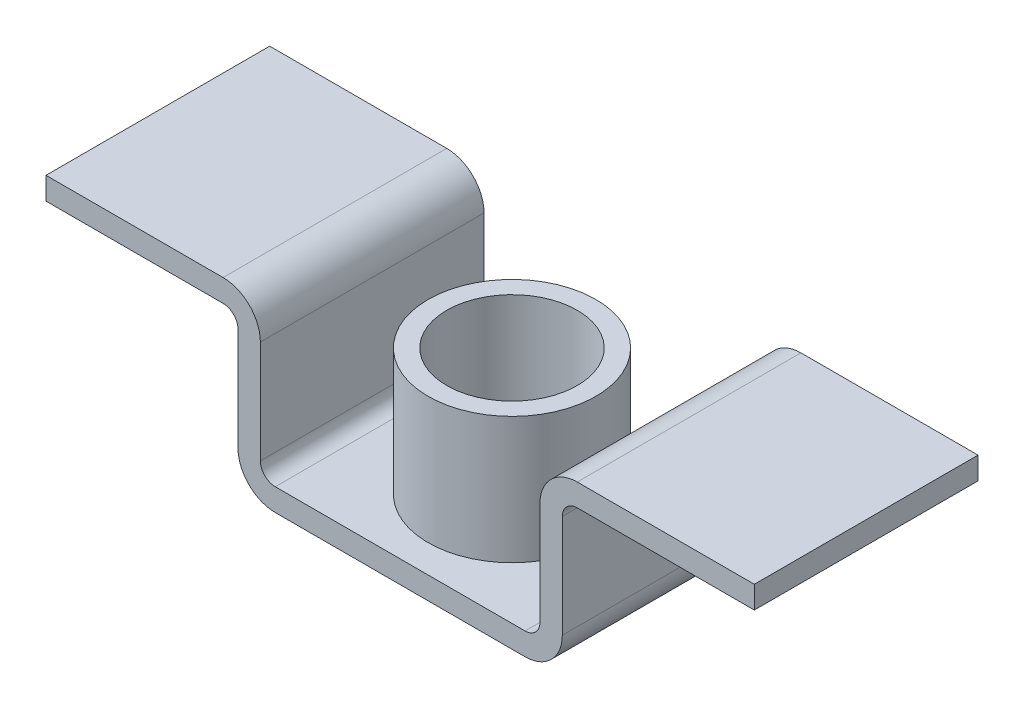
ISO-10303-21;
HEADER;
FILE_DESCRIPTION(('STEP AP214'),'2;1');
FILE_NAME('part.step','',(''),(''),'','','');
FILE_SCHEMA(('AUTOMOTIVE_DESIGN { 1 0 10303 214 1 1 1 1 }'));
ENDSEC;
DATA;
#1=APPLICATION_CONTEXT('core data for automotive mechanical design processes');
#2=APPLICATION_PROTOCOL_DEFINITION('international standard','automotive_design',2000,#1);
#3=PRODUCT_CONTEXT('',#1,'mechanical');
#4=PRODUCT('Part','Part','',(#3));
#5=PRODUCT_RELATED_PRODUCT_CATEGORY('part','',(#4));
#6=PRODUCT_DEFINITION_FORMATION('','',#4);
#7=PRODUCT_DEFINITION_CONTEXT('part definition',#1,'design');
#8=PRODUCT_DEFINITION('design','',#6,#7);
#9=PRODUCT_DEFINITION_SHAPE('','',#8);
#10=(LENGTH_UNIT() NAMED_UNIT(*) SI_UNIT(.MILLI.,.METRE.));
#11=(NAMED_UNIT(*) PLANE_ANGLE_UNIT() SI_UNIT($,.RADIAN.));
#12=(NAMED_UNIT(*) SI_UNIT($,.STERADIAN.) SOLID_ANGLE_UNIT());
#13=UNCERTAINTY_MEASURE_WITH_UNIT(LENGTH_MEASURE(1.E-05),#10,'distance_accuracy_value','');
#14=(GEOMETRIC_REPRESENTATION_CONTEXT(3) GLOBAL_UNCERTAINTY_ASSIGNED_CONTEXT((#13)) GLOBAL_UNIT_ASSIGNED_CONTEXT((#10,
#11,#12)) REPRESENTATION_CONTEXT('',''));
#15=CARTESIAN_POINT('',(0.,0.,0.));
#16=DIRECTION('',(0.,0.,1.));
#17=DIRECTION('',(1.,0.,0.));
#18=AXIS2_PLACEMENT_3D('',#15,#16,#17);
#19=CARTESIAN_POINT('',(-167.5,-188.,150.));
#20=DIRECTION('',(0.,0.,-1.));
#21=DIRECTION('',(-1.,0.,0.));
#22=AXIS2_PLACEMENT_3D('',#19,#20,#21);
#23=CYLINDRICAL_SURFACE('',#22,20.);
#24=CARTESIAN_POINT('',(-167.5,-188.,-150.));
#25=DIRECTION('',(0.,0.,1.));
#26=DIRECTION('',(1.,0.,0.));
#27=AXIS2_PLACEMENT_3D('',#24,#25,#26);
#28=CIRCLE('',#27,20.);
#29=CARTESIAN_POINT('',(-187.5,-188.,-150.));
#30=VERTEX_POINT('',#29);
#31=CARTESIAN_POINT('',(-167.5,-208.,-150.));
#32=VERTEX_POINT('',#31);
#33=EDGE_CURVE('E207',#30,#32,#28,.T.);
#34=ORIENTED_EDGE('',*,*,#33,.F.);
#35=DIRECTION('',(0.,0.,-1.));
#36=VECTOR('',#35,1.);
#37=CARTESIAN_POINT('',(-187.5,-188.,150.));
#38=LINE('',#37,#36);
#39=CARTESIAN_POINT('',(-187.5,-188.,150.));
#40=VERTEX_POINT('',#39);
#41=EDGE_CURVE('E50',#40,#30,#38,.T.);
#42=ORIENTED_EDGE('',*,*,#41,.F.);
#43=CARTESIAN_POINT('',(-167.5,-188.,150.));
#44=DIRECTION('',(0.,0.,1.));
#45=DIRECTION('',(1.,0.,0.));
#46=AXIS2_PLACEMENT_3D('',#43,#44,#45);
#47=CIRCLE('',#46,20.);
#48=CARTESIAN_POINT('',(-167.5,-208.,150.));
#49=VERTEX_POINT('',#48);
#50=EDGE_CURVE('E270',#40,#49,#47,.T.);
#51=ORIENTED_EDGE('',*,*,#50,.T.);
#52=DIRECTION('',(0.,0.,-1.));
#53=VECTOR('',#52,1.);
#54=CARTESIAN_POINT('',(-167.5,-208.,150.));
#55=LINE('',#54,#53);
#56=EDGE_CURVE('E133',#49,#32,#55,.T.);
#57=ORIENTED_EDGE('',*,*,#56,.T.);
#58=EDGE_LOOP('',(#34,#42,#51,#57));
#59=FACE_BOUND('',#58,.T.);
#60=ADVANCED_FACE('F39',(#59),#23,.F.);
#61=CARTESIAN_POINT('',(-187.5,-50.0000000000003,150.));
#62=DIRECTION('',(1.,0.,0.));
#63=DIRECTION('',(0.,1.,0.));
#64=AXIS2_PLACEMENT_3D('',#61,#62,#63);
#65=PLANE('',#64);
#66=DIRECTION('',(0.,-1.,0.));
#67=VECTOR('',#66,1.);
#68=CARTESIAN_POINT('',(-187.5,-50.0000000000003,-150.));
#69=LINE('',#68,#67);
#70=CARTESIAN_POINT('',(-187.5,-50.0000000000003,-150.));
#71=VERTEX_POINT('',#70);
#72=EDGE_CURVE('E262',#71,#30,#69,.T.);
#73=ORIENTED_EDGE('',*,*,#72,.F.);
#74=DIRECTION('',(0.,0.,-1.));
#75=VECTOR('',#74,1.);
#76=CARTESIAN_POINT('',(-187.5,-50.0000000000003,150.));
#77=LINE('',#76,#75);
#78=CARTESIAN_POINT('',(-187.5,-50.0000000000003,150.));
#79=VERTEX_POINT('',#78);
#80=EDGE_CURVE('E119',#79,#71,#77,.T.);
#81=ORIENTED_EDGE('',*,*,#80,.F.);
#82=DIRECTION('',(0.,-1.,0.));
#83=VECTOR('',#82,1.);
#84=CARTESIAN_POINT('',(-187.5,-50.0000000000003,150.));
#85=LINE('',#84,#83);
#86=EDGE_CURVE('E200',#79,#40,#85,.T.);
#87=ORIENTED_EDGE('',*,*,#86,.T.);
#88=ORIENTED_EDGE('',*,*,#41,.T.);
#89=EDGE_LOOP('',(#73,#81,#87,#88));
#90=FACE_BOUND('',#89,.T.);
#91=ADVANCED_FACE('F302',(#90),#65,.T.);
#92=CARTESIAN_POINT('',(-237.5,-50.,150.));
#93=DIRECTION('',(0.,0.,-1.));
#94=DIRECTION('',(-1.,0.,0.));
#95=AXIS2_PLACEMENT_3D('',#92,#93,#94);
#96=CYLINDRICAL_SURFACE('',#95,50.);
#97=CARTESIAN_POINT('',(-237.5,-50.,-150.));
#98=DIRECTION('',(0.,0.,-1.));
#99=DIRECTION('',(-1.,0.,0.));
#100=AXIS2_PLACEMENT_3D('',#97,#98,#99);
#101=CIRCLE('',#100,50.);
#102=CARTESIAN_POINT('',(-237.5,0.,-150.));
#103=VERTEX_POINT('',#102);
#104=EDGE_CURVE('E188',#103,#71,#101,.T.);
#105=ORIENTED_EDGE('',*,*,#104,.F.);
#106=DIRECTION('',(0.,0.,-1.));
#107=VECTOR('',#106,1.);
#108=CARTESIAN_POINT('',(-237.5,0.,150.));
#109=LINE('',#108,#107);
#110=CARTESIAN_POINT('',(-237.5,0.,150.));
#111=VERTEX_POINT('',#110);
#112=EDGE_CURVE('E182',#111,#103,#109,.T.);
#113=ORIENTED_EDGE('',*,*,#112,.F.);
#114=CARTESIAN_POINT('',(-237.5,-50.,150.));
#115=DIRECTION('',(0.,0.,-1.));
#116=DIRECTION('',(-1.,0.,0.));
#117=AXIS2_PLACEMENT_3D('',#114,#115,#116);
#118=CIRCLE('',#117,50.);
#119=EDGE_CURVE('E184',#111,#79,#118,.T.);
#120=ORIENTED_EDGE('',*,*,#119,.T.);
#121=ORIENTED_EDGE('',*,*,#80,.T.);
#122=EDGE_LOOP('',(#105,#113,#120,#121));
#123=FACE_BOUND('',#122,.T.);
#124=ADVANCED_FACE('F181',(#123),#96,.T.);
#125=CARTESIAN_POINT('',(-475.,0.,150.));
#126=DIRECTION('',(0.,1.,0.));
#127=DIRECTION('',(0.,0.,1.));
#128=AXIS2_PLACEMENT_3D('',#125,#126,#127);
#129=PLANE('',#128);
#130=DIRECTION('',(1.,0.,0.));
#131=VECTOR('',#130,1.);
#132=CARTESIAN_POINT('',(-475.,0.,-150.));
#133=LINE('',#132,#131);
#134=CARTESIAN_POINT('',(-475.,0.,-150.));
#135=VERTEX_POINT('',#134);
#136=EDGE_CURVE('E261',#135,#103,#133,.T.);
#137=ORIENTED_EDGE('',*,*,#136,.F.);
#138=DIRECTION('',(0.,0.,-1.));
#139=VECTOR('',#138,1.);
#140=CARTESIAN_POINT('',(-475.,0.,150.));
#141=LINE('',#140,#139);
#142=CARTESIAN_POINT('',(-475.,0.,150.));
#143=VERTEX_POINT('',#142);
#144=EDGE_CURVE('E193',#143,#135,#141,.T.);
#145=ORIENTED_EDGE('',*,*,#144,.F.);
#146=DIRECTION('',(1.,0.,0.));
#147=VECTOR('',#146,1.);
#148=CARTESIAN_POINT('',(-475.,0.,150.));
#149=LINE('',#148,#147);
#150=EDGE_CURVE('E197',#143,#111,#149,.T.);
#151=ORIENTED_EDGE('',*,*,#150,.T.);
#152=ORIENTED_EDGE('',*,*,#112,.T.);
#153=EDGE_LOOP('',(#137,#145,#151,#152));
#154=FACE_BOUND('',#153,.T.);
#155=ADVANCED_FACE('F203',(#154),#129,.T.);
#156=CARTESIAN_POINT('',(-475.,-30.,150.));
#157=DIRECTION('',(-1.,0.,0.));
#158=DIRECTION('',(0.,0.,1.));
#159=AXIS2_PLACEMENT_3D('',#156,#157,#158);
#160=PLANE('',#159);
#161=DIRECTION('',(0.,1.,0.));
#162=VECTOR('',#161,1.);
#163=CARTESIAN_POINT('',(-475.,-30.,-150.));
#164=LINE('',#163,#162);
#165=CARTESIAN_POINT('',(-475.,-30.,-150.));
#166=VERTEX_POINT('',#165);
#167=EDGE_CURVE('E256',#166,#135,#164,.T.);
#168=ORIENTED_EDGE('',*,*,#167,.F.);
#169=DIRECTION('',(0.,0.,-1.));
#170=VECTOR('',#169,1.);
#171=CARTESIAN_POINT('',(-475.,-30.,150.));
#172=LINE('',#171,#170);
#173=CARTESIAN_POINT('',(-475.,-30.,150.));
#174=VERTEX_POINT('',#173);
#175=EDGE_CURVE('E271',#174,#166,#172,.T.);
#176=ORIENTED_EDGE('',*,*,#175,.F.);
#177=DIRECTION('',(0.,1.,0.));
#178=VECTOR('',#177,1.);
#179=CARTESIAN_POINT('',(-475.,-30.,150.));
#180=LINE('',#179,#178);
#181=EDGE_CURVE('E205',#174,#143,#180,.T.);
#182=ORIENTED_EDGE('',*,*,#181,.T.);
#183=ORIENTED_EDGE('',*,*,#144,.T.);
#184=EDGE_LOOP('',(#168,#176,#182,#183));
#185=FACE_BOUND('',#184,.T.);
#186=ADVANCED_FACE('F320',(#185),#160,.T.);
#187=CARTESIAN_POINT('',(-237.5,-30.,150.));
#188=DIRECTION('',(0.,-1.,0.));
#189=DIRECTION('',(1.,0.,0.));
#190=AXIS2_PLACEMENT_3D('',#187,#188,#189);
#191=PLANE('',#190);
#192=DIRECTION('',(-1.,0.,0.));
#193=VECTOR('',#192,1.);
#194=CARTESIAN_POINT('',(-237.5,-30.,-150.));
#195=LINE('',#194,#193);
#196=CARTESIAN_POINT('',(-237.5,-30.,-150.));
#197=VERTEX_POINT('',#196);
#198=EDGE_CURVE('E254',#197,#166,#195,.T.);
#199=ORIENTED_EDGE('',*,*,#198,.F.);
#200=DIRECTION('',(0.,0.,-1.));
#201=VECTOR('',#200,1.);
#202=CARTESIAN_POINT('',(-237.5,-30.,150.));
#203=LINE('',#202,#201);
#204=CARTESIAN_POINT('',(-237.5,-30.,150.));
#205=VERTEX_POINT('',#204);
#206=EDGE_CURVE('E272',#205,#197,#203,.T.);
#207=ORIENTED_EDGE('',*,*,#206,.F.);
#208=DIRECTION('',(-1.,0.,0.));
#209=VECTOR('',#208,1.);
#210=CARTESIAN_POINT('',(-237.5,-30.,150.));
#211=LINE('',#210,#209);
#212=EDGE_CURVE('E204',#205,#174,#211,.T.);
#213=ORIENTED_EDGE('',*,*,#212,.T.);
#214=ORIENTED_EDGE('',*,*,#175,.T.);
#215=EDGE_LOOP('',(#199,#207,#213,#214));
#216=FACE_BOUND('',#215,.T.);
#217=ADVANCED_FACE('F319',(#216),#191,.T.);
#218=CARTESIAN_POINT('',(-237.5,-50.,150.));
#219=DIRECTION('',(0.,0.,-1.));
#220=DIRECTION('',(-1.,0.,0.));
#221=AXIS2_PLACEMENT_3D('',#218,#219,#220);
#222=CYLINDRICAL_SURFACE('',#221,20.);
#223=CARTESIAN_POINT('',(-237.5,-50.,-150.));
#224=DIRECTION('',(0.,0.,1.));
#225=DIRECTION('',(1.,0.,0.));
#226=AXIS2_PLACEMENT_3D('',#223,#224,#225);
#227=CIRCLE('',#226,20.);
#228=CARTESIAN_POINT('',(-217.5,-50.0000000000001,-150.));
#229=VERTEX_POINT('',#228);
#230=EDGE_CURVE('E252',#229,#197,#227,.T.);
#231=ORIENTED_EDGE('',*,*,#230,.F.);
#232=DIRECTION('',(0.,0.,-1.));
#233=VECTOR('',#232,1.);
#234=CARTESIAN_POINT('',(-217.5,-50.0000000000001,150.));
#235=LINE('',#234,#233);
#236=CARTESIAN_POINT('',(-217.5,-50.0000000000001,150.));
#237=VERTEX_POINT('',#236);
#238=EDGE_CURVE('E274',#237,#229,#235,.T.);
#239=ORIENTED_EDGE('',*,*,#238,.F.);
#240=CARTESIAN_POINT('',(-237.5,-50.,150.));
#241=DIRECTION('',(0.,0.,1.));
#242=DIRECTION('',(1.,0.,0.));
#243=AXIS2_PLACEMENT_3D('',#240,#241,#242);
#244=CIRCLE('',#243,20.);
#245=EDGE_CURVE('E460',#237,#205,#244,.T.);
#246=ORIENTED_EDGE('',*,*,#245,.T.);
#247=ORIENTED_EDGE('',*,*,#206,.T.);
#248=EDGE_LOOP('',(#231,#239,#246,#247));
#249=FACE_BOUND('',#248,.T.);
#250=ADVANCED_FACE('F322',(#249),#222,.F.);
#251=CARTESIAN_POINT('',(-217.5,-188.,150.));
#252=DIRECTION('',(-1.,0.,0.));
#253=DIRECTION('',(0.,0.,1.));
#254=AXIS2_PLACEMENT_3D('',#251,#252,#253);
#255=PLANE('',#254);
#256=DIRECTION('',(0.,1.,0.));
#257=VECTOR('',#256,1.);
#258=CARTESIAN_POINT('',(-217.5,-188.,-150.));
#259=LINE('',#258,#257);
#260=CARTESIAN_POINT('',(-217.5,-188.,-150.));
#261=VERTEX_POINT('',#260);
#262=EDGE_CURVE('E247',#261,#229,#259,.T.);
#263=ORIENTED_EDGE('',*,*,#262,.F.);
#264=DIRECTION('',(0.,0.,-1.));
#265=VECTOR('',#264,1.);
#266=CARTESIAN_POINT('',(-217.5,-188.,150.));
#267=LINE('',#266,#265);
#268=CARTESIAN_POINT('',(-217.5,-188.,150.));
#269=VERTEX_POINT('',#268);
#270=EDGE_CURVE('E280',#269,#261,#267,.T.);
#271=ORIENTED_EDGE('',*,*,#270,.F.);
#272=DIRECTION('',(0.,1.,0.));
#273=VECTOR('',#272,1.);
#274=CARTESIAN_POINT('',(-217.5,-188.,150.));
#275=LINE('',#274,#273);
#276=EDGE_CURVE('E452',#269,#237,#275,.T.);
#277=ORIENTED_EDGE('',*,*,#276,.T.);
#278=ORIENTED_EDGE('',*,*,#238,.T.);
#279=EDGE_LOOP('',(#263,#271,#277,#278));
#280=FACE_BOUND('',#279,.T.);
#281=ADVANCED_FACE('F327',(#280),#255,.T.);
#282=CARTESIAN_POINT('',(-167.5,-188.,150.));
#283=DIRECTION('',(0.,0.,-1.));
#284=DIRECTION('',(-1.,0.,0.));
#285=AXIS2_PLACEMENT_3D('',#282,#283,#284);
#286=CYLINDRICAL_SURFACE('',#285,50.);
#287=CARTESIAN_POINT('',(-167.5,-188.,-150.));
#288=DIRECTION('',(0.,0.,-1.));
#289=DIRECTION('',(-1.,0.,0.));
#290=AXIS2_PLACEMENT_3D('',#287,#288,#289);
#291=CIRCLE('',#290,50.);
#292=CARTESIAN_POINT('',(-167.5,-238.,-150.));
#293=VERTEX_POINT('',#292);
#294=EDGE_CURVE('E248',#293,#261,#291,.T.);
#295=ORIENTED_EDGE('',*,*,#294,.F.);
#296=DIRECTION('',(0.,0.,-1.));
#297=VECTOR('',#296,1.);
#298=CARTESIAN_POINT('',(-167.5,-238.,150.));
#299=LINE('',#298,#297);
#300=CARTESIAN_POINT('',(-167.5,-238.,150.));
#301=VERTEX_POINT('',#300);
#302=EDGE_CURVE('E276',#301,#293,#299,.T.);
#303=ORIENTED_EDGE('',*,*,#302,.F.);
#304=CARTESIAN_POINT('',(-167.5,-188.,150.));
#305=DIRECTION('',(0.,0.,-1.));
#306=DIRECTION('',(-1.,0.,0.));
#307=AXIS2_PLACEMENT_3D('',#304,#305,#306);
#308=CIRCLE('',#307,50.);
#309=EDGE_CURVE('E453',#301,#269,#308,.T.);
#310=ORIENTED_EDGE('',*,*,#309,.T.);
#311=ORIENTED_EDGE('',*,*,#270,.T.);
#312=EDGE_LOOP('',(#295,#303,#310,#311));
#313=FACE_BOUND('',#312,.T.);
#314=ADVANCED_FACE('F335',(#313),#286,.T.);
#315=CARTESIAN_POINT('',(167.5,-238.,150.));
#316=DIRECTION('',(0.,-1.,0.));
#317=DIRECTION('',(1.,0.,0.));
#318=AXIS2_PLACEMENT_3D('',#315,#316,#317);
#319=PLANE('',#318);
#320=CARTESIAN_POINT('',(0.,-238.,0.));
#321=DIRECTION('',(0.,-1.,0.));
#322=DIRECTION('',(1.,0.,0.));
#323=AXIS2_PLACEMENT_3D('',#320,#321,#322);
#324=CIRCLE('',#323,37.5);
#325=CARTESIAN_POINT('',(37.5,-238.,0.));
#326=VERTEX_POINT('',#325);
#327=EDGE_CURVE('E408',#326,#326,#324,.F.);
#328=ORIENTED_EDGE('',*,*,#327,.T.);
#329=EDGE_LOOP('',(#328));
#330=FACE_BOUND('',#329,.T.);
#331=DIRECTION('',(-1.,0.,0.));
#332=VECTOR('',#331,1.);
#333=CARTESIAN_POINT('',(167.5,-238.,-150.));
#334=LINE('',#333,#332);
#335=CARTESIAN_POINT('',(167.5,-238.,-150.));
#336=VERTEX_POINT('',#335);
#337=EDGE_CURVE('E241',#336,#293,#334,.T.);
#338=ORIENTED_EDGE('',*,*,#337,.F.);
#339=DIRECTION('',(0.,0.,-1.));
#340=VECTOR('',#339,1.);
#341=CARTESIAN_POINT('',(167.5,-238.,150.));
#342=LINE('',#341,#340);
#343=CARTESIAN_POINT('',(167.5,-238.,150.));
#344=VERTEX_POINT('',#343);
#345=EDGE_CURVE('E283',#344,#336,#342,.T.);
#346=ORIENTED_EDGE('',*,*,#345,.F.);
#347=DIRECTION('',(-1.,0.,0.));
#348=VECTOR('',#347,1.);
#349=CARTESIAN_POINT('',(167.5,-238.,150.));
#350=LINE('',#349,#348);
#351=EDGE_CURVE('E446',#344,#301,#350,.T.);
#352=ORIENTED_EDGE('',*,*,#351,.T.);
#353=ORIENTED_EDGE('',*,*,#302,.T.);
#354=EDGE_LOOP('',(#338,#346,#352,#353));
#355=FACE_BOUND('',#354,.T.);
#356=ADVANCED_FACE('F338',(#330,#355),#319,.T.);
#357=CARTESIAN_POINT('',(167.5,-188.,150.));
#358=DIRECTION('',(0.,0.,-1.));
#359=DIRECTION('',(-1.,0.,0.));
#360=AXIS2_PLACEMENT_3D('',#357,#358,#359);
#361=CYLINDRICAL_SURFACE('',#360,50.);
#362=CARTESIAN_POINT('',(167.5,-188.,-150.));
#363=DIRECTION('',(0.,0.,-1.));
#364=DIRECTION('',(-1.,0.,0.));
#365=AXIS2_PLACEMENT_3D('',#362,#363,#364);
#366=CIRCLE('',#365,50.);
#367=CARTESIAN_POINT('',(217.5,-188.,-150.));
#368=VERTEX_POINT('',#367);
#369=EDGE_CURVE('E238',#368,#336,#366,.T.);
#370=ORIENTED_EDGE('',*,*,#369,.F.);
#371=DIRECTION('',(0.,0.,-1.));
#372=VECTOR('',#371,1.);
#373=CARTESIAN_POINT('',(217.5,-188.,150.));
#374=LINE('',#373,#372);
#375=CARTESIAN_POINT('',(217.5,-188.,150.));
#376=VERTEX_POINT('',#375);
#377=EDGE_CURVE('E281',#376,#368,#374,.T.);
#378=ORIENTED_EDGE('',*,*,#377,.F.);
#379=CARTESIAN_POINT('',(167.5,-188.,150.));
#380=DIRECTION('',(0.,0.,-1.));
#381=DIRECTION('',(-1.,0.,0.));
#382=AXIS2_PLACEMENT_3D('',#379,#380,#381);
#383=CIRCLE('',#382,50.);
#384=EDGE_CURVE('E443',#376,#344,#383,.T.);
#385=ORIENTED_EDGE('',*,*,#384,.T.);
#386=ORIENTED_EDGE('',*,*,#345,.T.);
#387=EDGE_LOOP('',(#370,#378,#385,#386));
#388=FACE_BOUND('',#387,.T.);
#389=ADVANCED_FACE('F337',(#388),#361,.T.);
#390=CARTESIAN_POINT('',(217.5,-50.0000000000001,150.));
#391=DIRECTION('',(1.,0.,0.));
#392=DIRECTION('',(0.,1.,0.));
#393=AXIS2_PLACEMENT_3D('',#390,#391,#392);
#394=PLANE('',#393);
#395=DIRECTION('',(0.,-1.,0.));
#396=VECTOR('',#395,1.);
#397=CARTESIAN_POINT('',(217.5,-50.0000000000001,-150.));
#398=LINE('',#397,#396);
#399=CARTESIAN_POINT('',(217.5,-50.,-150.));
#400=VERTEX_POINT('',#399);
#401=EDGE_CURVE('E240',#400,#368,#398,.T.);
#402=ORIENTED_EDGE('',*,*,#401,.F.);
#403=DIRECTION('',(0.,0.,-1.));
#404=VECTOR('',#403,1.);
#405=CARTESIAN_POINT('',(217.5,-50.,150.));
#406=LINE('',#405,#404);
#407=CARTESIAN_POINT('',(217.5,-50.,150.));
#408=VERTEX_POINT('',#407);
#409=EDGE_CURVE('E282',#408,#400,#406,.T.);
#410=ORIENTED_EDGE('',*,*,#409,.F.);
#411=DIRECTION('',(0.,-1.,0.));
#412=VECTOR('',#411,1.);
#413=CARTESIAN_POINT('',(217.5,-50.0000000000001,150.));
#414=LINE('',#413,#412);
#415=EDGE_CURVE('E445',#408,#376,#414,.T.);
#416=ORIENTED_EDGE('',*,*,#415,.T.);
#417=ORIENTED_EDGE('',*,*,#377,.T.);
#418=EDGE_LOOP('',(#402,#410,#416,#417));
#419=FACE_BOUND('',#418,.T.);
#420=ADVANCED_FACE('F342',(#419),#394,.T.);
#421=CARTESIAN_POINT('',(237.5,-49.9999999999999,150.));
#422=DIRECTION('',(0.,0.,-1.));
#423=DIRECTION('',(-1.,0.,0.));
#424=AXIS2_PLACEMENT_3D('',#421,#422,#423);
#425=CYLINDRICAL_SURFACE('',#424,20.);
#426=CARTESIAN_POINT('',(237.5,-49.9999999999999,-150.));
#427=DIRECTION('',(0.,0.,1.));
#428=DIRECTION('',(1.,0.,0.));
#429=AXIS2_PLACEMENT_3D('',#426,#427,#428);
#430=CIRCLE('',#429,20.);
#431=CARTESIAN_POINT('',(237.5,-29.9999999999999,-150.));
#432=VERTEX_POINT('',#431);
#433=EDGE_CURVE('E232',#432,#400,#430,.T.);
#434=ORIENTED_EDGE('',*,*,#433,.F.);
#435=DIRECTION('',(0.,0.,-1.));
#436=VECTOR('',#435,1.);
#437=CARTESIAN_POINT('',(237.5,-29.9999999999999,150.));
#438=LINE('',#437,#436);
#439=CARTESIAN_POINT('',(237.5,-29.9999999999999,150.));
#440=VERTEX_POINT('',#439);
#441=EDGE_CURVE('E290',#440,#432,#438,.T.);
#442=ORIENTED_EDGE('',*,*,#441,.F.);
#443=CARTESIAN_POINT('',(237.5,-49.9999999999999,150.));
#444=DIRECTION('',(0.,0.,1.));
#445=DIRECTION('',(1.,0.,0.));
#446=AXIS2_PLACEMENT_3D('',#443,#444,#445);
#447=CIRCLE('',#446,20.);
#448=EDGE_CURVE('E438',#440,#408,#447,.T.);
#449=ORIENTED_EDGE('',*,*,#448,.T.);
#450=ORIENTED_EDGE('',*,*,#409,.T.);
#451=EDGE_LOOP('',(#434,#442,#449,#450));
#452=FACE_BOUND('',#451,.T.);
#453=ADVANCED_FACE('F346',(#452),#425,.F.);
#454=CARTESIAN_POINT('',(475.,-29.9999999999999,150.));
#455=DIRECTION('',(0.,-1.,0.));
#456=DIRECTION('',(1.,0.,0.));
#457=AXIS2_PLACEMENT_3D('',#454,#455,#456);
#458=PLANE('',#457);
#459=DIRECTION('',(-1.,0.,0.));
#460=VECTOR('',#459,1.);
#461=CARTESIAN_POINT('',(475.,-29.9999999999999,-150.));
#462=LINE('',#461,#460);
#463=CARTESIAN_POINT('',(475.,-29.9999999999999,-150.));
#464=VERTEX_POINT('',#463);
#465=EDGE_CURVE('E233',#464,#432,#462,.T.);
#466=ORIENTED_EDGE('',*,*,#465,.F.);
#467=DIRECTION('',(0.,0.,-1.));
#468=VECTOR('',#467,1.);
#469=CARTESIAN_POINT('',(475.,-29.9999999999999,150.));
#470=LINE('',#469,#468);
#471=CARTESIAN_POINT('',(475.,-29.9999999999999,150.));
#472=VERTEX_POINT('',#471);
#473=EDGE_CURVE('E287',#472,#464,#470,.T.);
#474=ORIENTED_EDGE('',*,*,#473,.F.);
#475=DIRECTION('',(-1.,0.,0.));
#476=VECTOR('',#475,1.);
#477=CARTESIAN_POINT('',(475.,-29.9999999999999,150.));
#478=LINE('',#477,#476);
#479=EDGE_CURVE('E436',#472,#440,#478,.T.);
#480=ORIENTED_EDGE('',*,*,#479,.T.);
#481=ORIENTED_EDGE('',*,*,#441,.T.);
#482=EDGE_LOOP('',(#466,#474,#480,#481));
#483=FACE_BOUND('',#482,.T.);
#484=ADVANCED_FACE('F355',(#483),#458,.T.);
#485=CARTESIAN_POINT('',(475.,1.16341445918999E-13,150.));
#486=DIRECTION('',(1.,0.,0.));
#487=DIRECTION('',(0.,0.,-1.));
#488=AXIS2_PLACEMENT_3D('',#485,#486,#487);
#489=PLANE('',#488);
#490=DIRECTION('',(0.,-1.,0.));
#491=VECTOR('',#490,1.);
#492=CARTESIAN_POINT('',(475.,1.16341445918999E-13,-150.));
#493=LINE('',#492,#491);
#494=CARTESIAN_POINT('',(475.,1.16341445918999E-13,-150.));
#495=VERTEX_POINT('',#494);
#496=EDGE_CURVE('E226',#495,#464,#493,.T.);
#497=ORIENTED_EDGE('',*,*,#496,.F.);
#498=DIRECTION('',(0.,0.,-1.));
#499=VECTOR('',#498,1.);
#500=CARTESIAN_POINT('',(475.,1.16341445918999E-13,150.));
#501=LINE('',#500,#499);
#502=CARTESIAN_POINT('',(475.,1.16341445918999E-13,150.));
#503=VERTEX_POINT('',#502);
#504=EDGE_CURVE('E292',#503,#495,#501,.T.);
#505=ORIENTED_EDGE('',*,*,#504,.F.);
#506=DIRECTION('',(0.,-1.,0.));
#507=VECTOR('',#506,1.);
#508=CARTESIAN_POINT('',(475.,1.16341445918999E-13,150.));
#509=LINE('',#508,#507);
#510=EDGE_CURVE('E433',#503,#472,#509,.T.);
#511=ORIENTED_EDGE('',*,*,#510,.T.);
#512=ORIENTED_EDGE('',*,*,#473,.T.);
#513=EDGE_LOOP('',(#497,#505,#511,#512));
#514=FACE_BOUND('',#513,.T.);
#515=ADVANCED_FACE('F358',(#514),#489,.T.);
#516=CARTESIAN_POINT('',(237.5,0.,150.));
#517=DIRECTION('',(0.,1.,0.));
#518=DIRECTION('',(-1.,0.,0.));
#519=AXIS2_PLACEMENT_3D('',#516,#517,#518);
#520=PLANE('',#519);
#521=DIRECTION('',(1.,0.,0.));
#522=VECTOR('',#521,1.);
#523=CARTESIAN_POINT('',(237.5,0.,-150.));
#524=LINE('',#523,#522);
#525=CARTESIAN_POINT('',(237.5,0.,-150.));
#526=VERTEX_POINT('',#525);
#527=EDGE_CURVE('E223',#526,#495,#524,.T.);
#528=ORIENTED_EDGE('',*,*,#527,.F.);
#529=DIRECTION('',(0.,0.,-1.));
#530=VECTOR('',#529,1.);
#531=CARTESIAN_POINT('',(237.5,0.,150.));
#532=LINE('',#531,#530);
#533=CARTESIAN_POINT('',(237.5,0.,150.));
#534=VERTEX_POINT('',#533);
#535=EDGE_CURVE('E291',#534,#526,#532,.T.);
#536=ORIENTED_EDGE('',*,*,#535,.F.);
#537=DIRECTION('',(1.,0.,0.));
#538=VECTOR('',#537,1.);
#539=CARTESIAN_POINT('',(237.5,0.,150.));
#540=LINE('',#539,#538);
#541=EDGE_CURVE('E429',#534,#503,#540,.T.);
#542=ORIENTED_EDGE('',*,*,#541,.T.);
#543=ORIENTED_EDGE('',*,*,#504,.T.);
#544=EDGE_LOOP('',(#528,#536,#542,#543));
#545=FACE_BOUND('',#544,.T.);
#546=ADVANCED_FACE('F359',(#545),#520,.T.);
#547=CARTESIAN_POINT('',(237.5,-50.,150.));
#548=DIRECTION('',(0.,0.,-1.));
#549=DIRECTION('',(-1.,0.,0.));
#550=AXIS2_PLACEMENT_3D('',#547,#548,#549);
#551=CYLINDRICAL_SURFACE('',#550,50.);
#552=CARTESIAN_POINT('',(237.5,-50.,-150.));
#553=DIRECTION('',(0.,0.,-1.));
#554=DIRECTION('',(-1.,0.,0.));
#555=AXIS2_PLACEMENT_3D('',#552,#553,#554);
#556=CIRCLE('',#555,50.);
#557=CARTESIAN_POINT('',(187.5,-50.0000000000003,-150.));
#558=VERTEX_POINT('',#557);
#559=EDGE_CURVE('E225',#558,#526,#556,.T.);
#560=ORIENTED_EDGE('',*,*,#559,.F.);
#561=DIRECTION('',(0.,0.,-1.));
#562=VECTOR('',#561,1.);
#563=CARTESIAN_POINT('',(187.5,-50.0000000000003,150.));
#564=LINE('',#563,#562);
#565=CARTESIAN_POINT('',(187.5,-50.0000000000003,150.));
#566=VERTEX_POINT('',#565);
#567=EDGE_CURVE('E293',#566,#558,#564,.T.);
#568=ORIENTED_EDGE('',*,*,#567,.F.);
#569=CARTESIAN_POINT('',(237.5,-50.,150.));
#570=DIRECTION('',(0.,0.,-1.));
#571=DIRECTION('',(-1.,0.,0.));
#572=AXIS2_PLACEMENT_3D('',#569,#570,#571);
#573=CIRCLE('',#572,50.);
#574=EDGE_CURVE('E430',#566,#534,#573,.T.);
#575=ORIENTED_EDGE('',*,*,#574,.T.);
#576=ORIENTED_EDGE('',*,*,#535,.T.);
#577=EDGE_LOOP('',(#560,#568,#575,#576));
#578=FACE_BOUND('',#577,.T.);
#579=ADVANCED_FACE('F365',(#578),#551,.T.);
#580=CARTESIAN_POINT('',(187.5,-188.,150.));
#581=DIRECTION('',(-1.,0.,0.));
#582=DIRECTION('',(0.,-1.,0.));
#583=AXIS2_PLACEMENT_3D('',#580,#581,#582);
#584=PLANE('',#583);
#585=DIRECTION('',(0.,1.,0.));
#586=VECTOR('',#585,1.);
#587=CARTESIAN_POINT('',(187.5,-188.,-150.));
#588=LINE('',#587,#586);
#589=CARTESIAN_POINT('',(187.5,-188.,-150.));
#590=VERTEX_POINT('',#589);
#591=EDGE_CURVE('E218',#590,#558,#588,.T.);
#592=ORIENTED_EDGE('',*,*,#591,.F.);
#593=DIRECTION('',(0.,0.,-1.));
#594=VECTOR('',#593,1.);
#595=CARTESIAN_POINT('',(187.5,-188.,150.));
#596=LINE('',#595,#594);
#597=CARTESIAN_POINT('',(187.5,-188.,150.));
#598=VERTEX_POINT('',#597);
#599=EDGE_CURVE('E300',#598,#590,#596,.T.);
#600=ORIENTED_EDGE('',*,*,#599,.F.);
#601=DIRECTION('',(0.,1.,0.));
#602=VECTOR('',#601,1.);
#603=CARTESIAN_POINT('',(187.5,-188.,150.));
#604=LINE('',#603,#602);
#605=EDGE_CURVE('E424',#598,#566,#604,.T.);
#606=ORIENTED_EDGE('',*,*,#605,.T.);
#607=ORIENTED_EDGE('',*,*,#567,.T.);
#608=EDGE_LOOP('',(#592,#600,#606,#607));
#609=FACE_BOUND('',#608,.T.);
#610=ADVANCED_FACE('F366',(#609),#584,.T.);
#611=CARTESIAN_POINT('',(167.5,-188.,150.));
#612=DIRECTION('',(0.,0.,-1.));
#613=DIRECTION('',(-1.,0.,0.));
#614=AXIS2_PLACEMENT_3D('',#611,#612,#613);
#615=CYLINDRICAL_SURFACE('',#614,20.);
#616=CARTESIAN_POINT('',(167.5,-188.,-150.));
#617=DIRECTION('',(0.,0.,1.));
#618=DIRECTION('',(1.,0.,0.));
#619=AXIS2_PLACEMENT_3D('',#616,#617,#618);
#620=CIRCLE('',#619,20.);
#621=CARTESIAN_POINT('',(167.5,-208.,-150.));
#622=VERTEX_POINT('',#621);
#623=EDGE_CURVE('E216',#622,#590,#620,.T.);
#624=ORIENTED_EDGE('',*,*,#623,.F.);
#625=DIRECTION('',(0.,0.,-1.));
#626=VECTOR('',#625,1.);
#627=CARTESIAN_POINT('',(167.5,-208.,150.));
#628=LINE('',#627,#626);
#629=CARTESIAN_POINT('',(167.5,-208.,150.));
#630=VERTEX_POINT('',#629);
#631=EDGE_CURVE('E299',#630,#622,#628,.T.);
#632=ORIENTED_EDGE('',*,*,#631,.F.);
#633=CARTESIAN_POINT('',(167.5,-188.,150.));
#634=DIRECTION('',(0.,0.,1.));
#635=DIRECTION('',(1.,0.,0.));
#636=AXIS2_PLACEMENT_3D('',#633,#634,#635);
#637=CIRCLE('',#636,20.);
#638=EDGE_CURVE('E423',#630,#598,#637,.T.);
#639=ORIENTED_EDGE('',*,*,#638,.T.);
#640=ORIENTED_EDGE('',*,*,#599,.T.);
#641=EDGE_LOOP('',(#624,#632,#639,#640));
#642=FACE_BOUND('',#641,.T.);
#643=ADVANCED_FACE('F375',(#642),#615,.F.);
#644=CARTESIAN_POINT('',(-167.5,-208.,150.));
#645=DIRECTION('',(0.,1.,0.));
#646=DIRECTION('',(-1.,0.,0.));
#647=AXIS2_PLACEMENT_3D('',#644,#645,#646);
#648=PLANE('',#647);
#649=CARTESIAN_POINT('',(0.,-208.,0.));
#650=DIRECTION('',(0.,1.,0.));
#651=DIRECTION('',(-1.,0.,0.));
#652=AXIS2_PLACEMENT_3D('',#649,#650,#651);
#653=CIRCLE('',#652,112.5);
#654=CARTESIAN_POINT('',(-112.5,-208.,0.));
#655=VERTEX_POINT('',#654);
#656=EDGE_CURVE('E409',#655,#655,#653,.T.);
#657=ORIENTED_EDGE('',*,*,#656,.F.);
#658=EDGE_LOOP('',(#657));
#659=FACE_BOUND('',#658,.T.);
#660=DIRECTION('',(1.,0.,0.));
#661=VECTOR('',#660,1.);
#662=CARTESIAN_POINT('',(-167.5,-208.,-150.));
#663=LINE('',#662,#661);
#664=EDGE_CURVE('E215',#32,#622,#663,.T.);
#665=ORIENTED_EDGE('',*,*,#664,.F.);
#666=ORIENTED_EDGE('',*,*,#56,.F.);
#667=DIRECTION('',(1.,0.,0.));
#668=VECTOR('',#667,1.);
#669=CARTESIAN_POINT('',(-167.5,-208.,150.));
#670=LINE('',#669,#668);
#671=EDGE_CURVE('E420',#49,#630,#670,.T.);
#672=ORIENTED_EDGE('',*,*,#671,.T.);
#673=ORIENTED_EDGE('',*,*,#631,.T.);
#674=EDGE_LOOP('',(#665,#666,#672,#673));
#675=FACE_BOUND('',#674,.T.);
#676=ADVANCED_FACE('F297',(#659,#675),#648,.T.);
#677=CARTESIAN_POINT('',(-167.5,-188.,150.));
#678=DIRECTION('',(0.,0.,1.));
#679=DIRECTION('',(1.,0.,0.));
#680=AXIS2_PLACEMENT_3D('',#677,#678,#679);
#681=PLANE('',#680);
#682=ORIENTED_EDGE('',*,*,#50,.F.);
#683=ORIENTED_EDGE('',*,*,#86,.F.);
#684=ORIENTED_EDGE('',*,*,#119,.F.);
#685=ORIENTED_EDGE('',*,*,#150,.F.);
#686=ORIENTED_EDGE('',*,*,#181,.F.);
#687=ORIENTED_EDGE('',*,*,#212,.F.);
#688=ORIENTED_EDGE('',*,*,#245,.F.);
#689=ORIENTED_EDGE('',*,*,#276,.F.);
#690=ORIENTED_EDGE('',*,*,#309,.F.);
#691=ORIENTED_EDGE('',*,*,#351,.F.);
#692=ORIENTED_EDGE('',*,*,#384,.F.);
#693=ORIENTED_EDGE('',*,*,#415,.F.);
#694=ORIENTED_EDGE('',*,*,#448,.F.);
#695=ORIENTED_EDGE('',*,*,#479,.F.);
#696=ORIENTED_EDGE('',*,*,#510,.F.);
#697=ORIENTED_EDGE('',*,*,#541,.F.);
#698=ORIENTED_EDGE('',*,*,#574,.F.);
#699=ORIENTED_EDGE('',*,*,#605,.F.);
#700=ORIENTED_EDGE('',*,*,#638,.F.);
#701=ORIENTED_EDGE('',*,*,#671,.F.);
#702=EDGE_LOOP('',(#682,#683,#684,#685,#686,#687,#688,#689,#690,#691,#692,#693,#694,#695,#696,
#697,#698,#699,#700,#701));
#703=FACE_BOUND('',#702,.T.);
#704=ADVANCED_FACE('F194',(#703),#681,.T.);
#705=CARTESIAN_POINT('',(-167.5,-188.,-150.));
#706=DIRECTION('',(0.,0.,1.));
#707=DIRECTION('',(1.,0.,0.));
#708=AXIS2_PLACEMENT_3D('',#705,#706,#707);
#709=PLANE('',#708);
#710=ORIENTED_EDGE('',*,*,#33,.T.);
#711=ORIENTED_EDGE('',*,*,#664,.T.);
#712=ORIENTED_EDGE('',*,*,#623,.T.);
#713=ORIENTED_EDGE('',*,*,#591,.T.);
#714=ORIENTED_EDGE('',*,*,#559,.T.);
#715=ORIENTED_EDGE('',*,*,#527,.T.);
#716=ORIENTED_EDGE('',*,*,#496,.T.);
#717=ORIENTED_EDGE('',*,*,#465,.T.);
#718=ORIENTED_EDGE('',*,*,#433,.T.);
#719=ORIENTED_EDGE('',*,*,#401,.T.);
#720=ORIENTED_EDGE('',*,*,#369,.T.);
#721=ORIENTED_EDGE('',*,*,#337,.T.);
#722=ORIENTED_EDGE('',*,*,#294,.T.);
#723=ORIENTED_EDGE('',*,*,#262,.T.);
#724=ORIENTED_EDGE('',*,*,#230,.T.);
#725=ORIENTED_EDGE('',*,*,#198,.T.);
#726=ORIENTED_EDGE('',*,*,#167,.T.);
#727=ORIENTED_EDGE('',*,*,#136,.T.);
#728=ORIENTED_EDGE('',*,*,#104,.T.);
#729=ORIENTED_EDGE('',*,*,#72,.T.);
#730=EDGE_LOOP('',(#710,#711,#712,#713,#714,#715,#716,#717,#718,#719,#720,#721,#722,#723,#724,
#725,#726,#727,#728,#729));
#731=FACE_BOUND('',#730,.T.);
#732=ADVANCED_FACE('F301',(#731),#709,.F.);
#733=CARTESIAN_POINT('',(0.,-38.,0.));
#734=DIRECTION('',(0.,1.,0.));
#735=DIRECTION('',(-1.,0.,0.));
#736=AXIS2_PLACEMENT_3D('',#733,#734,#735);
#737=PLANE('',#736);
#738=CARTESIAN_POINT('',(0.,-38.,0.));
#739=DIRECTION('',(0.,1.,0.));
#740=DIRECTION('',(-1.,0.,0.));
#741=AXIS2_PLACEMENT_3D('',#738,#739,#740);
#742=CIRCLE('',#741,112.5);
#743=CARTESIAN_POINT('',(-112.5,-38.,0.));
#744=VERTEX_POINT('',#743);
#745=EDGE_CURVE('E213',#744,#744,#742,.T.);
#746=ORIENTED_EDGE('',*,*,#745,.T.);
#747=EDGE_LOOP('',(#746));
#748=FACE_BOUND('',#747,.T.);
#749=CARTESIAN_POINT('',(0.,-38.,0.));
#750=DIRECTION('',(0.,1.,0.));
#751=DIRECTION('',(-1.,0.,0.));
#752=AXIS2_PLACEMENT_3D('',#749,#750,#751);
#753=CIRCLE('',#752,87.5);
#754=CARTESIAN_POINT('',(-87.5,-38.,0.));
#755=VERTEX_POINT('',#754);
#756=EDGE_CURVE('E403',#755,#755,#753,.T.);
#757=ORIENTED_EDGE('',*,*,#756,.F.);
#758=EDGE_LOOP('',(#757));
#759=FACE_BOUND('',#758,.T.);
#760=ADVANCED_FACE('F491',(#748,#759),#737,.T.);
#761=CARTESIAN_POINT('',(0.,-38.,0.));
#762=DIRECTION('',(0.,-1.,0.));
#763=DIRECTION('',(1.,0.,0.));
#764=AXIS2_PLACEMENT_3D('',#761,#762,#763);
#765=CYLINDRICAL_SURFACE('',#764,112.5);
#766=ORIENTED_EDGE('',*,*,#745,.F.);
#767=EDGE_LOOP('',(#766));
#768=FACE_BOUND('',#767,.T.);
#769=ORIENTED_EDGE('',*,*,#656,.T.);
#770=EDGE_LOOP('',(#769));
#771=FACE_BOUND('',#770,.T.);
#772=ADVANCED_FACE('F392',(#768,#771),#765,.T.);
#773=CARTESIAN_POINT('',(0.,-38.,0.));
#774=DIRECTION('',(0.,-1.,0.));
#775=DIRECTION('',(1.,0.,0.));
#776=AXIS2_PLACEMENT_3D('',#773,#774,#775);
#777=CYLINDRICAL_SURFACE('',#776,87.5);
#778=ORIENTED_EDGE('',*,*,#756,.T.);
#779=EDGE_LOOP('',(#778));
#780=FACE_BOUND('',#779,.T.);
#781=CARTESIAN_POINT('',(0.,-208.,0.));
#782=DIRECTION('',(0.,1.,0.));
#783=DIRECTION('',(-1.,0.,0.));
#784=AXIS2_PLACEMENT_3D('',#781,#782,#783);
#785=CIRCLE('',#784,87.5);
#786=CARTESIAN_POINT('',(-87.5,-208.,0.));
#787=VERTEX_POINT('',#786);
#788=EDGE_CURVE('E11',#787,#787,#785,.F.);
#789=ORIENTED_EDGE('',*,*,#788,.T.);
#790=EDGE_LOOP('',(#789));
#791=FACE_BOUND('',#790,.T.);
#792=ADVANCED_FACE('F390',(#780,#791),#777,.F.);
#793=CARTESIAN_POINT('',(0.,-208.,0.));
#794=DIRECTION('',(0.,1.,0.));
#795=DIRECTION('',(-1.,0.,0.));
#796=AXIS2_PLACEMENT_3D('',#793,#794,#795);
#797=CIRCLE('',#796,37.5);
#798=CARTESIAN_POINT('',(-37.5,-208.,0.));
#799=VERTEX_POINT('',#798);
#800=EDGE_CURVE('E402',#799,#799,#797,.T.);
#801=ORIENTED_EDGE('',*,*,#800,.F.);
#802=EDGE_LOOP('',(#801));
#803=FACE_BOUND('',#802,.T.);
#804=ORIENTED_EDGE('',*,*,#788,.F.);
#805=EDGE_LOOP('',(#804));
#806=FACE_BOUND('',#805,.T.);
#807=ADVANCED_FACE('F378',(#803,#806),#648,.T.);
#808=CARTESIAN_POINT('',(0.,-238.001,0.));
#809=DIRECTION('',(0.,1.,0.));
#810=DIRECTION('',(-1.,0.,0.));
#811=AXIS2_PLACEMENT_3D('',#808,#809,#810);
#812=CYLINDRICAL_SURFACE('',#811,37.5);
#813=ORIENTED_EDGE('',*,*,#327,.F.);
#814=EDGE_LOOP('',(#813));
#815=FACE_BOUND('',#814,.T.);
#816=ORIENTED_EDGE('',*,*,#800,.T.);
#817=EDGE_LOOP('',(#816));
#818=FACE_BOUND('',#817,.T.);
#819=ADVANCED_FACE('F387',(#815,#818),#812,.F.);
#820=CLOSED_SHELL('',(#60,#91,#124,#155,#186,#217,#250,#281,#314,#356,#389,#420,#453,#484,#515,
#546,#579,#610,#643,#676,#704,#732,#760,#772,#792,#807,#819));
#821=MANIFOLD_SOLID_BREP('B2',#820);
#822=ADVANCED_BREP_SHAPE_REPRESENTATION('',(#18,#821),#14);
#823=SHAPE_DEFINITION_REPRESENTATION(#9,#822);
ENDSEC;
END-ISO-10303-21;
